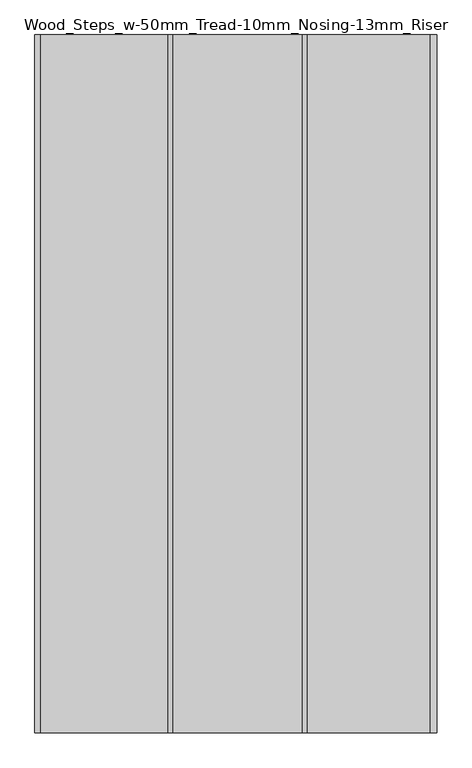
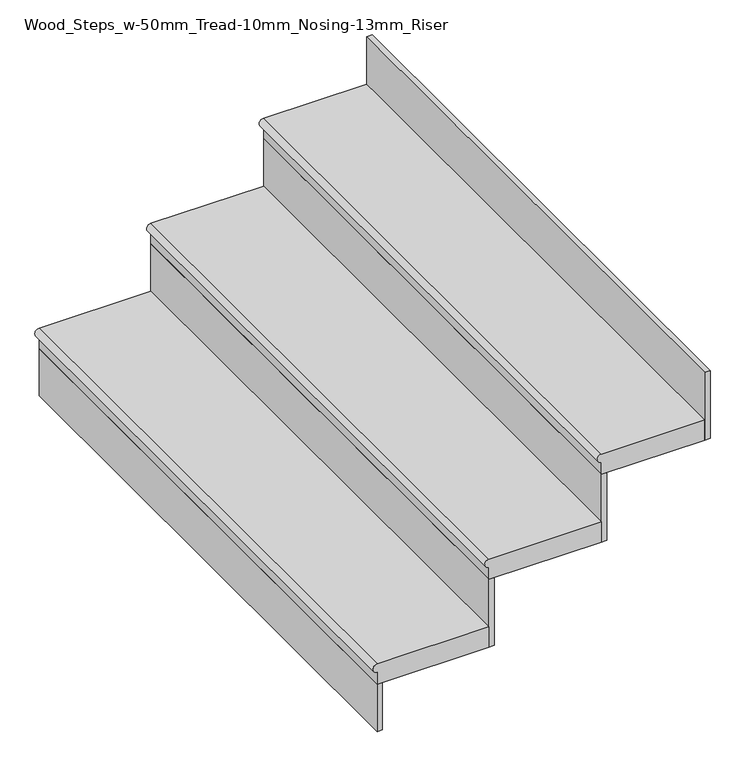
"""IFC4 building model written with IfcOpenShell, lengths in millimetres: stair flight geometry, Wood_Steps_w-50mm_Tread-10mm_Nosing-13mm_Riser."""

from ifc_helpers import new_model, si_unit, point, frame, frame_2d, origin, origin_with_axes, place, context, project, spatial, polyline, circle_curve, trimmed, segment, composite_curve, outline, extrude, source, transform, mapped, element, save


def wood_steps_w_50mm_tread_10mm_nosing_13mm_riser_0e3a26d2(model_context):
    return source(origin(), model_context, "Body", "SweptSolid", [
        extrude(outline(composite_curve([segment(polyline([(166.6666667, -5746.6079187), (166.6666667, -6006.6079187)]), True, "CONTINUOUS"), segment(trimmed(circle_curve(frame_2d((156.6666667, -6006.6079187)), 10.0), [point((166.6666667, -6006.6079187))], [point((146.6666667, -6006.6079187))], False, "CARTESIAN"), True, "CONTINUOUS"), segment(polyline([(146.6666667, -6006.6079187), (116.6666667, -6006.6079187), (116.6666667, -5746.6079187), (166.6666667, -5746.6079187)]), True, "CONTINUOUS")], self_intersect=False)), frame((0.0, 5786.998858, 0.0), z_axis=(0.0, 1.0, 0.0), x_axis=(0.0, 0.0, 1.0)), (0.0, 0.0, 1.0), 1361.1074494),
        extrude(outline(polyline([(-5994.1079187, 5786.998858), (-6006.6079187, 5786.998858), (-6006.6079187, 7148.1063074), (-5994.1079187, 7148.1063074), (-5994.1079187, 5786.998858)])), origin_with_axes(), (0.0, 0.0, 1.0), 116.6666667),
        extrude(outline(polyline([(-5734.1079187, 5786.998858), (-5746.6079187, 5786.998858), (-5746.6079187, 7148.1063074), (-5734.1079187, 7148.1063074), (-5734.1079187, 5786.998858)])), frame((0.0, 0.0, 116.6666667), z_axis=(0.0, 0.0, 1.0), x_axis=(1.0, 0.0, 0.0)), (0.0, 0.0, 1.0), 166.6666667),
        extrude(outline(composite_curve([segment(polyline([(333.3333333, -5484.8904087), (333.3333333, -5746.6079187)]), True, "CONTINUOUS"), segment(trimmed(circle_curve(frame_2d((323.3333333, -5746.6079187)), 10.0), [point((333.3333333, -5746.6079187))], [point((313.3333333, -5746.6079187))], False, "CARTESIAN"), True, "CONTINUOUS"), segment(polyline([(313.3333333, -5746.6079187), (283.3333333, -5746.6079187), (283.3333333, -5484.8904087), (333.3333333, -5484.8904087)]), True, "CONTINUOUS")], self_intersect=False)), frame((0.0, 5786.998858, 0.0), z_axis=(0.0, 1.0, 0.0), x_axis=(0.0, 0.0, 1.0)), (0.0, 0.0, 1.0), 1361.1074494),
        extrude(outline(polyline([(-5472.3904087, 5786.998858), (-5484.8904087, 5786.998858), (-5484.8904087, 7148.1063074), (-5472.3904087, 7148.1063074), (-5472.3904087, 5786.998858)])), frame((0.0, 0.0, 283.3333333), z_axis=(0.0, 0.0, 1.0), x_axis=(1.0, 0.0, 0.0)), (0.0, 0.0, 1.0), 166.6666667),
        extrude(outline(polyline([(-5232.3904087, 5786.998858), (-5244.8904087, 5786.998858), (-5244.8904087, 7148.1063074), (-5232.3904087, 7148.1063074), (-5232.3904087, 5786.998858)])), frame((0.0, 0.0, 450.0), z_axis=(0.0, 0.0, 1.0), x_axis=(1.0, 0.0, 0.0)), (0.0, 0.0, 1.0), 166.6666667),
        extrude(outline(composite_curve([segment(polyline([(500.0, -5244.8904087), (500.0, -5484.8904087)]), True, "CONTINUOUS"), segment(trimmed(circle_curve(frame_2d((490.0, -5484.8904087)), 10.0), [point((500.0, -5484.8904087))], [point((480.0, -5484.8904087))], False, "CARTESIAN"), True, "CONTINUOUS"), segment(polyline([(480.0, -5484.8904087), (450.0, -5484.8904087), (450.0, -5244.8904087), (500.0, -5244.8904087)]), True, "CONTINUOUS")], self_intersect=False)), frame((0.0, 5786.998858, 0.0), z_axis=(0.0, 1.0, 0.0), x_axis=(0.0, 0.0, 1.0)), (0.0, 0.0, 1.0), 1361.1074494),
    ])


if __name__ == "__main__":
    model = new_model("IFC4")
    model_context = context("Model", 3, world=origin())
    ifc_project = project(units=[si_unit("LENGTHUNIT", "METRE", prefix="MILLI")], contexts=[model_context])
    site = spatial("IfcSite", under=ifc_project)
    building = spatial("IfcBuilding", under=site)
    placement = place(None, origin())
    wood_steps_w_50mm_tread_10mm_nosing_13mm_riser_shape = wood_steps_w_50mm_tread_10mm_nosing_13mm_riser_0e3a26d2(model_context)
    element("IfcStairFlight", 1, ObjectType="Wood_Steps_w-50mm_Tread-10mm_Nosing-13mm_Riser", at=placement, inside=building, context=model_context, shape_type="MappedRepresentation", body=[
        mapped(wood_steps_w_50mm_tread_10mm_nosing_13mm_riser_shape, transform((0.0, 0.0, 0.0), x_axis=(1.0, 0.0, 0.0), y_axis=(0.0, 1.0, 0.0), z_axis=(0.0, 0.0, 1.0))),
    ])
    save(model, "model.ifc")

# Revit data of these elements
# Element 1 (IfcStairFlight, "Wood_Steps_w-50mm_Tread-10mm_Nosing-13mm_Riser")
#   Materials on its faces: "Oak Flooring"
# Materials
#   "Oak Flooring": class "Wood", colour RGB 212 179 113, transparency 0, Description = "Quercus Rubra", Cost = 0
